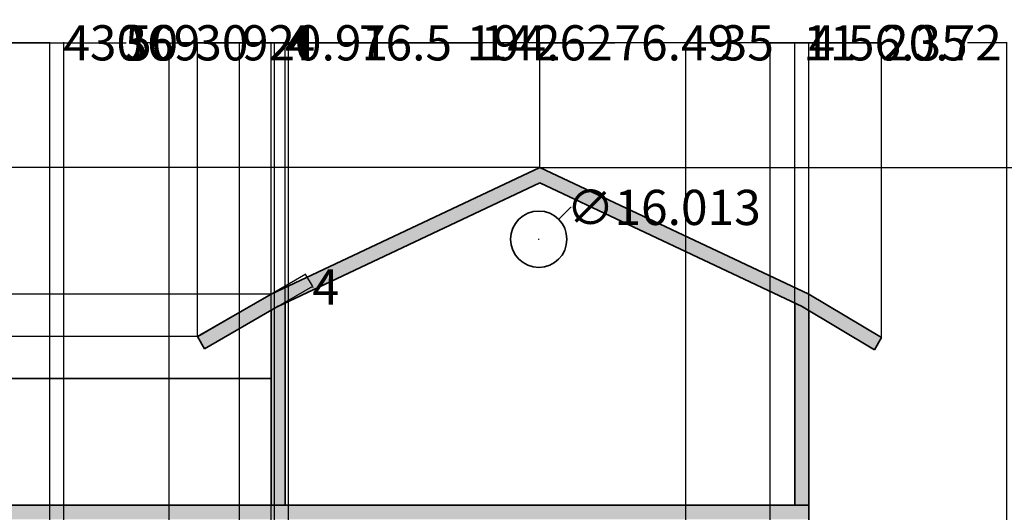
# Model space of a CAD drawing. Units: inches. Extents: x 403 to 1256, y 451 to 842.
# Tile 3 of 4: x 818 to 1098, y 702 to 842. Entities that reach past the tile are written whole.
import ezdxf

# ---------------------------------------------------------------- set-up
doc = ezdxf.new("R2010")
doc.units = ezdxf.units.IN
doc.header["$MEASUREMENT"] = 0
for name, color, linetype, lineweight in [('A-ANNO-DIMS', 2, 'Continuous', 18), ('A-ROOF', 30, 'Continuous', 35), ('A-ROOF-PATT', 30, 'Continuous', 13), ('A-WALL', 7, 'Continuous', 35), ('A-WALL-PATT', 8, 'Continuous', 13)]:
    doc.layers.add(name, color=color, linetype=linetype, lineweight=lineweight)
doc.styles.get("Standard").update_dxf_attribs({"font": 'arial.ttf'})
doc.dimstyles.get("Standard").update_dxf_attribs({"dimtxt": 10, "dimasz": 0.18, "dimexe": 0.18, "dimexo": 0.0625, "dimgap": 0.09, "dimtad": 0, "dimtih": 1, "dimtoh": 1, "dimdec": 0, "dimzin": 0, "dimdsep": 46, "dimlunit": 3, "dimtxsty": 'Standard', "dimcen": 0.09, "dimadec": 0, "dimazin": 0, "dimtfac": 1, "dimtdec": 0, "dimtofl": 0, "dimtmove": 0, "dimatfit": 3, "dimfxl": 1, "dimtolj": 1, "dimtzin": 0, "dimarcsym": 0})

# ---------------------------------------------------------------- blocks, each defined once
blk = doc.blocks.new('*D11')
at = {"layer": 'A-ANNO-DIMS', "color": 0, "lineweight": -2, "transparency": 16777216}
for p, q in [((673.46, 704.02), (673.46, 835.54)), ((673.64, 835.36), (846.82, 835.36)), ((1042.28, 835.36), (869.1, 835.36)), ((1042.46, 704.02), (1042.46, 835.54))]:
    blk.add_line(p, q, dxfattribs=at)
at = {"layer": 'A-ANNO-DIMS', "color": 0, "transparency": 16777216}
for points in [[(673.64, 835.39), (673.64, 835.33), (673.46, 835.36)], [(1042.28, 835.39), (1042.28, 835.33), (1042.46, 835.36)]]:
    blk.add_solid(points, dxfattribs=at)
at = {"layer": 'Defpoints', "color": 0, "transparency": 16777216}
for p in [(1042.46, 835.36), (673.46, 703.96), (1042.46, 703.96)]:
    blk.add_point(p, dxfattribs=at)
at = {"layer": 'A-ANNO-DIMS', "color": 0, "transparency": 16777216, "insert": (857.96, 835.36), "char_height": 10, "attachment_point": 5}
blk.add_mtext('\\A1;369', dxfattribs=at)
blk = doc.blocks.new('*D12')
at = {"layer": 'A-ANNO-DIMS', "color": 0, "lineweight": -2, "transparency": 16777216}
for p, q in [((966.02, 799.96), (1244.44, 799.96)), ((1244.26, 799.78), (1244.26, 632.66)), ((1244.26, 455.14), (1244.26, 622.26)), ((1042.52, 454.96), (1244.44, 454.96))]:
    blk.add_line(p, q, dxfattribs=at)
at = {"layer": 'A-ANNO-DIMS', "color": 0, "transparency": 16777216}
for points in [[(1244.23, 799.78), (1244.29, 799.78), (1244.26, 799.96)], [(1244.23, 455.14), (1244.29, 455.14), (1244.26, 454.96)]]:
    blk.add_solid(points, dxfattribs=at)
at = {"layer": 'Defpoints', "color": 0, "transparency": 16777216}
for p in [(965.96, 799.96), (1244.26, 799.96), (1042.46, 454.96)]:
    blk.add_point(p, dxfattribs=at)
at = {"layer": 'A-ANNO-DIMS', "color": 0, "transparency": 16777216, "insert": (1244.26, 627.46), "char_height": 10, "attachment_point": 5}
blk.add_mtext('\\A1;345', dxfattribs=at)
blk = doc.blocks.new('*D18')
at = {"layer": 'A-ANNO-DIMS', "color": 0, "lineweight": -2, "transparency": 16777216}
for p, q in [((965.9, 799.96), (473.5, 799.96)), ((473.68, 799.78), (473.68, 775.16)), ((473.68, 740.14), (473.68, 764.77)), ((673.4, 739.96), (473.5, 739.96))]:
    blk.add_line(p, q, dxfattribs=at)
at = {"layer": 'A-ANNO-DIMS', "color": 0, "transparency": 16777216}
for points in [[(473.65, 799.78), (473.71, 799.78), (473.68, 799.96)], [(473.65, 740.14), (473.71, 740.14), (473.68, 739.96)]]:
    blk.add_solid(points, dxfattribs=at)
at = {"layer": 'Defpoints', "color": 0, "transparency": 16777216}
for p in [(473.68, 799.96), (965.96, 799.96), (673.46, 739.96)]:
    blk.add_point(p, dxfattribs=at)
at = {"layer": 'A-ANNO-DIMS', "color": 0, "transparency": 16777216, "insert": (473.68, 769.96), "char_height": 10, "attachment_point": 5}
blk.add_mtext('\\A1;60', dxfattribs=at)
blk = doc.blocks.new('*D22')
at = {"layer": 'A-ANNO-DIMS', "color": 0, "lineweight": -2, "transparency": 16777216}
for p, q in [((1007.46, 616.02), (1007.46, 835.54)), ((1007.64, 835.36), (1017.67, 835.36)), ((1042.28, 835.36), (1032.25, 835.36)), ((1042.46, 704.02), (1042.46, 835.54))]:
    blk.add_line(p, q, dxfattribs=at)
at = {"layer": 'A-ANNO-DIMS', "color": 0, "transparency": 16777216}
for points in [[(1007.64, 835.39), (1007.64, 835.33), (1007.46, 835.36)], [(1042.28, 835.39), (1042.28, 835.33), (1042.46, 835.36)]]:
    blk.add_solid(points, dxfattribs=at)
at = {"layer": 'Defpoints', "color": 0, "transparency": 16777216}
for p in [(1042.46, 835.36), (1042.46, 703.96), (1007.46, 615.96)]:
    blk.add_point(p, dxfattribs=at)
at = {"layer": 'A-ANNO-DIMS', "color": 0, "transparency": 16777216, "insert": (1024.96, 835.36), "char_height": 10, "attachment_point": 5}
blk.add_mtext('\\A1;35', dxfattribs=at)
blk = doc.blocks.new('*D23')
at = {"layer": 'A-ANNO-DIMS', "color": 0, "lineweight": -2, "transparency": 16777216}
for p, q in [((682.46, 455.02), (682.46, 835.54)), ((682.64, 835.36), (743.81, 835.36)), ((826.28, 835.36), (765.1, 835.36)), ((826.46, 455.02), (826.46, 835.54))]:
    blk.add_line(p, q, dxfattribs=at)
at = {"layer": 'A-ANNO-DIMS', "color": 0, "transparency": 16777216}
for points in [[(682.64, 835.39), (682.64, 835.33), (682.46, 835.36)], [(826.28, 835.39), (826.28, 835.33), (826.46, 835.36)]]:
    blk.add_solid(points, dxfattribs=at)
at = {"layer": 'Defpoints', "color": 0, "transparency": 16777216}
for p in [(826.46, 835.36), (682.46, 454.96), (826.46, 454.96)]:
    blk.add_point(p, dxfattribs=at)
at = {"layer": 'A-ANNO-DIMS', "color": 0, "transparency": 16777216, "insert": (754.46, 835.36), "char_height": 10, "attachment_point": 5}
blk.add_mtext('\\A1;144', dxfattribs=at)
blk = doc.blocks.new('*D24')
at = {"layer": 'A-ANNO-DIMS', "color": 0, "lineweight": -2, "transparency": 16777216}
for p, q in [((830.46, 539.02), (830.46, 835.54)), ((830.64, 835.36), (848.22, 835.36)), ((880.28, 835.36), (862.69, 835.36)), ((880.46, 539.02), (880.46, 835.54))]:
    blk.add_line(p, q, dxfattribs=at)
at = {"layer": 'A-ANNO-DIMS', "color": 0, "transparency": 16777216}
for points in [[(830.64, 835.39), (830.64, 835.33), (830.46, 835.36)], [(880.28, 835.39), (880.28, 835.33), (880.46, 835.36)]]:
    blk.add_solid(points, dxfattribs=at)
at = {"layer": 'Defpoints', "color": 0, "transparency": 16777216}
for p in [(880.46, 835.36), (830.46, 538.96), (880.46, 538.96)]:
    blk.add_point(p, dxfattribs=at)
at = {"layer": 'A-ANNO-DIMS', "color": 0, "transparency": 16777216, "insert": (855.46, 835.36), "char_height": 10, "attachment_point": 5}
blk.add_mtext('\\A1;50', dxfattribs=at)
blk = doc.blocks.new('*D25')
at = {"layer": 'A-ANNO-DIMS', "color": 0, "lineweight": -2, "transparency": 16777216}
for p, q in [((889.46, 539.02), (889.46, 835.54)), ((889.64, 835.36), (949.84, 835.36)), ((1031.28, 835.36), (971.07, 835.36)), ((1031.46, 539.02), (1031.46, 835.54))]:
    blk.add_line(p, q, dxfattribs=at)
at = {"layer": 'A-ANNO-DIMS', "color": 0, "transparency": 16777216}
for points in [[(889.64, 835.39), (889.64, 835.33), (889.46, 835.36)], [(1031.28, 835.39), (1031.28, 835.33), (1031.46, 835.36)]]:
    blk.add_solid(points, dxfattribs=at)
at = {"layer": 'Defpoints', "color": 0, "transparency": 16777216}
for p in [(1031.46, 835.36), (889.46, 538.96), (1031.46, 538.96)]:
    blk.add_point(p, dxfattribs=at)
at = {"layer": 'A-ANNO-DIMS', "color": 0, "transparency": 16777216, "insert": (960.46, 835.36), "char_height": 10, "attachment_point": 5}
blk.add_mtext('\\A1;142', dxfattribs=at)
blk = doc.blocks.new('*D26')
at = {"layer": 'A-ANNO-DIMS', "color": 0, "lineweight": -2, "transparency": 16777216}
for p, q in [((880.46, 539.02), (880.46, 835.54)), ((880.64, 835.36), (881.58, 835.36)), ((889.28, 835.36), (888.34, 835.36)), ((889.46, 539.02), (889.46, 835.54))]:
    blk.add_line(p, q, dxfattribs=at)
at = {"layer": 'A-ANNO-DIMS', "color": 0, "transparency": 16777216}
for points in [[(880.64, 835.39), (880.64, 835.33), (880.46, 835.36)], [(889.28, 835.39), (889.28, 835.33), (889.46, 835.36)]]:
    blk.add_solid(points, dxfattribs=at)
at = {"layer": 'Defpoints', "color": 0, "transparency": 16777216}
for p in [(889.46, 835.36), (880.46, 538.96), (889.46, 538.96)]:
    blk.add_point(p, dxfattribs=at)
at = {"layer": 'A-ANNO-DIMS', "color": 0, "transparency": 16777216, "insert": (884.96, 835.36), "char_height": 10, "attachment_point": 5}
blk.add_mtext('\\A1;9', dxfattribs=at)
blk = doc.blocks.new('*D27')
at = {"layer": 'A-ANNO-DIMS', "color": 0, "lineweight": -2, "transparency": 16777216}
for p, q in [((1031.46, 455.02), (1031.46, 835.54)), ((1031.64, 835.36), (1042.28, 835.36)), ((1042.46, 455.02), (1042.46, 835.54)), ((1042.46, 835.36), (1042.64, 835.36))]:
    blk.add_line(p, q, dxfattribs=at)
at = {"layer": 'A-ANNO-DIMS', "color": 0, "transparency": 16777216}
for points in [[(1031.64, 835.39), (1031.64, 835.33), (1031.46, 835.36)], [(1042.28, 835.39), (1042.28, 835.33), (1042.46, 835.36)]]:
    blk.add_solid(points, dxfattribs=at)
at = {"layer": 'Defpoints', "color": 0, "transparency": 16777216}
for p in [(1042.46, 835.36), (1031.46, 454.96), (1042.46, 454.96)]:
    blk.add_point(p, dxfattribs=at)
at = {"layer": 'A-ANNO-DIMS', "color": 0, "transparency": 16777216, "insert": (1048.46, 835.36), "char_height": 10, "attachment_point": 5}
blk.add_mtext('\\A1;11', dxfattribs=at)
blk = doc.blocks.new('*D30')
at = {"layer": 'A-ANNO-DIMS', "color": 0, "lineweight": -2, "transparency": 16777216}
for p, q in [((1042.46, 455.02), (1042.46, 835.54)), ((1042.64, 835.36), (1053.63, 835.36)), ((1098.63, 835.36), (1087.63, 835.36)), ((1098.81, 455.02), (1098.81, 835.54))]:
    blk.add_line(p, q, dxfattribs=at)
at = {"layer": 'A-ANNO-DIMS', "color": 0, "transparency": 16777216}
for points in [[(1042.64, 835.39), (1042.64, 835.33), (1042.46, 835.36)], [(1098.63, 835.39), (1098.63, 835.33), (1098.81, 835.36)]]:
    blk.add_solid(points, dxfattribs=at)
at = {"layer": 'Defpoints', "color": 0, "transparency": 16777216}
for p in [(1098.81, 835.36), (1042.46, 454.96), (1098.81, 454.96)]:
    blk.add_point(p, dxfattribs=at)
at = {"layer": 'A-ANNO-DIMS', "color": 0, "transparency": 16777216, "insert": (1070.63, 835.36), "char_height": 10, "attachment_point": 5}
blk.add_mtext('\\A1;56.35', dxfattribs=at)
blk = doc.blocks.new('*D35')
at = {"layer": 'A-ANNO-DIMS', "color": 0, "lineweight": -2, "transparency": 16777216}
for p, q in [((826.46, 616.02), (826.46, 835.54)), ((826.64, 835.36), (830.28, 835.36)), ((830.46, 616.02), (830.46, 835.54)), ((830.46, 835.36), (830.64, 835.36))]:
    blk.add_line(p, q, dxfattribs=at)
at = {"layer": 'A-ANNO-DIMS', "color": 0, "transparency": 16777216}
for points in [[(826.64, 835.39), (826.64, 835.33), (826.46, 835.36)], [(830.28, 835.39), (830.28, 835.33), (830.46, 835.36)]]:
    blk.add_solid(points, dxfattribs=at)
at = {"layer": 'Defpoints', "color": 0, "transparency": 16777216}
for p in [(830.46, 835.36), (826.46, 615.96), (830.46, 615.96)]:
    blk.add_point(p, dxfattribs=at)
at = {"layer": 'A-ANNO-DIMS', "color": 0, "transparency": 16777216, "insert": (834.19, 835.36), "char_height": 10, "attachment_point": 5}
blk.add_mtext('\\A1;4', dxfattribs=at)
blk = doc.blocks.new('*D36')
at = {"layer": 'A-ANNO-DIMS', "color": 0, "lineweight": -2, "transparency": 16777216}
for p, q in [((830.46, 616.02), (830.46, 835.54)), ((830.64, 835.36), (838.23, 835.36)), ((860.28, 835.36), (852.69, 835.36)), ((860.46, 616.02), (860.46, 835.54))]:
    blk.add_line(p, q, dxfattribs=at)
at = {"layer": 'A-ANNO-DIMS', "color": 0, "transparency": 16777216}
for points in [[(830.64, 835.39), (830.64, 835.33), (830.46, 835.36)], [(860.28, 835.39), (860.28, 835.33), (860.46, 835.36)]]:
    blk.add_solid(points, dxfattribs=at)
at = {"layer": 'Defpoints', "color": 0, "transparency": 16777216}
for p in [(860.46, 835.36), (830.46, 615.96), (860.46, 615.96)]:
    blk.add_point(p, dxfattribs=at)
at = {"layer": 'A-ANNO-DIMS', "color": 0, "transparency": 16777216, "insert": (845.46, 835.36), "char_height": 10, "attachment_point": 5}
blk.add_mtext('\\A1;30', dxfattribs=at)
blk = doc.blocks.new('*D37')
at = {"layer": 'A-ANNO-DIMS', "color": 0, "lineweight": -2, "transparency": 16777216}
for p, q in [((860.46, 656.02), (860.46, 835.54)), ((860.64, 835.36), (868.23, 835.36)), ((890.28, 835.36), (882.69, 835.36)), ((890.46, 656.02), (890.46, 835.54))]:
    blk.add_line(p, q, dxfattribs=at)
at = {"layer": 'A-ANNO-DIMS', "color": 0, "transparency": 16777216}
for points in [[(860.64, 835.39), (860.64, 835.33), (860.46, 835.36)], [(890.28, 835.39), (890.28, 835.33), (890.46, 835.36)]]:
    blk.add_solid(points, dxfattribs=at)
at = {"layer": 'Defpoints', "color": 0, "transparency": 16777216}
for p in [(890.46, 835.36), (860.46, 655.96), (890.46, 655.96)]:
    blk.add_point(p, dxfattribs=at)
at = {"layer": 'A-ANNO-DIMS', "color": 0, "transparency": 16777216, "insert": (875.46, 835.36), "char_height": 10, "attachment_point": 5}
blk.add_mtext('\\A1;30', dxfattribs=at)
blk = doc.blocks.new('*D38')
at = {"layer": 'A-ANNO-DIMS', "color": 0, "lineweight": -2, "transparency": 16777216}
for p, q in [((890.46, 616.02), (890.46, 835.54)), ((890.64, 835.36), (894.28, 835.36)), ((894.46, 616.02), (894.46, 835.54)), ((894.46, 835.36), (894.64, 835.36))]:
    blk.add_line(p, q, dxfattribs=at)
at = {"layer": 'A-ANNO-DIMS', "color": 0, "transparency": 16777216}
for points in [[(890.64, 835.39), (890.64, 835.33), (890.46, 835.36)], [(894.28, 835.39), (894.28, 835.33), (894.46, 835.36)]]:
    blk.add_solid(points, dxfattribs=at)
at = {"layer": 'Defpoints', "color": 0, "transparency": 16777216}
for p in [(894.46, 835.36), (890.46, 615.96), (894.46, 615.96)]:
    blk.add_point(p, dxfattribs=at)
at = {"layer": 'A-ANNO-DIMS', "color": 0, "transparency": 16777216, "insert": (898.19, 835.36), "char_height": 10, "attachment_point": 5}
blk.add_mtext('\\A1;4', dxfattribs=at)
blk = doc.blocks.new('*D43')
at = {"layer": 'A-ANNO-DIMS', "color": 0, "lineweight": -2, "transparency": 16777216}
for p, q in [((868.55, 751.96), (868.55, 835.54)), ((868.73, 835.36), (945.54, 835.36)), ((1062.99, 835.36), (986.19, 835.36)), ((1063.17, 751.65), (1063.17, 835.54))]:
    blk.add_line(p, q, dxfattribs=at)
at = {"layer": 'A-ANNO-DIMS', "color": 0, "transparency": 16777216}
for points in [[(868.73, 835.39), (868.73, 835.33), (868.55, 835.36)], [(1062.99, 835.39), (1062.99, 835.33), (1063.17, 835.36)]]:
    blk.add_solid(points, dxfattribs=at)
at = {"layer": 'Defpoints', "color": 0, "transparency": 16777216}
for p in [(1063.17, 835.36), (868.55, 751.9), (1063.17, 751.58)]:
    blk.add_point(p, dxfattribs=at)
at = {"layer": 'A-ANNO-DIMS', "color": 0, "transparency": 16777216, "insert": (965.86, 835.36), "char_height": 10, "attachment_point": 5}
blk.add_mtext('\\A1;194.62', dxfattribs=at)
blk = doc.blocks.new('*D44')
at = {"layer": 'A-ANNO-DIMS', "color": 0, "lineweight": -2, "transparency": 16777216}
for p, q in [((868.55, 751.96), (868.55, 835.54)), ((868.73, 835.36), (889.28, 835.36)), ((889.46, 764.02), (889.46, 835.54)), ((889.46, 835.36), (889.64, 835.36))]:
    blk.add_line(p, q, dxfattribs=at)
at = {"layer": 'A-ANNO-DIMS', "color": 0, "transparency": 16777216}
for points in [[(868.73, 835.39), (868.73, 835.33), (868.55, 835.36)], [(889.28, 835.39), (889.28, 835.33), (889.46, 835.36)]]:
    blk.add_solid(points, dxfattribs=at)
at = {"layer": 'Defpoints', "color": 0, "transparency": 16777216}
for p in [(889.46, 835.36), (889.46, 763.96), (868.55, 751.9)]:
    blk.add_point(p, dxfattribs=at)
at = {"layer": 'A-ANNO-DIMS', "color": 0, "transparency": 16777216, "insert": (905.72, 835.36), "char_height": 10, "attachment_point": 5}
blk.add_mtext('\\A1;20.91', dxfattribs=at)
blk = doc.blocks.new('*D45')
at = {"layer": 'A-ANNO-DIMS', "color": 0, "lineweight": -2, "transparency": 16777216}
for p, q in [((889.46, 764.02), (889.46, 835.54)), ((889.64, 835.36), (914.63, 835.36)), ((965.78, 835.36), (940.78, 835.36)), ((965.96, 800.02), (965.96, 835.54))]:
    blk.add_line(p, q, dxfattribs=at)
at = {"layer": 'A-ANNO-DIMS', "color": 0, "transparency": 16777216}
for points in [[(889.64, 835.39), (889.64, 835.33), (889.46, 835.36)], [(965.78, 835.39), (965.78, 835.33), (965.96, 835.36)]]:
    blk.add_solid(points, dxfattribs=at)
at = {"layer": 'Defpoints', "color": 0, "transparency": 16777216}
for p in [(965.96, 835.36), (965.96, 799.96), (889.46, 763.96)]:
    blk.add_point(p, dxfattribs=at)
at = {"layer": 'A-ANNO-DIMS', "color": 0, "transparency": 16777216, "insert": (927.71, 835.36), "char_height": 10, "attachment_point": 5}
blk.add_mtext('\\A1;76.5', dxfattribs=at)
blk = doc.blocks.new('*D46')
at = {"layer": 'A-ANNO-DIMS', "color": 0, "lineweight": -2, "transparency": 16777216}
for p, q in [((965.96, 800.02), (965.96, 835.54)), ((966.14, 835.36), (987.27, 835.36)), ((1042.27, 835.36), (1021.14, 835.36)), ((1042.45, 764.03), (1042.45, 835.54))]:
    blk.add_line(p, q, dxfattribs=at)
at = {"layer": 'A-ANNO-DIMS', "color": 0, "transparency": 16777216}
for points in [[(966.14, 835.39), (966.14, 835.33), (965.96, 835.36)], [(1042.27, 835.39), (1042.27, 835.33), (1042.45, 835.36)]]:
    blk.add_solid(points, dxfattribs=at)
at = {"layer": 'Defpoints', "color": 0, "transparency": 16777216}
for p in [(1042.45, 835.36), (965.96, 799.96), (1042.45, 763.97)]:
    blk.add_point(p, dxfattribs=at)
at = {"layer": 'A-ANNO-DIMS', "color": 0, "transparency": 16777216, "insert": (1004.2, 835.36), "char_height": 10, "attachment_point": 5}
blk.add_mtext('\\A1;76.49', dxfattribs=at)
blk = doc.blocks.new('*D47')
at = {"layer": 'A-ANNO-DIMS', "color": 0, "lineweight": -2, "transparency": 16777216}
for p, q in [((1042.45, 764.03), (1042.45, 835.54)), ((1042.63, 835.36), (1062.99, 835.36)), ((1063.17, 751.65), (1063.17, 835.54)), ((1063.17, 835.36), (1063.35, 835.36))]:
    blk.add_line(p, q, dxfattribs=at)
at = {"layer": 'A-ANNO-DIMS', "color": 0, "transparency": 16777216}
for points in [[(1042.63, 835.39), (1042.63, 835.33), (1042.45, 835.36)], [(1062.99, 835.39), (1062.99, 835.33), (1063.17, 835.36)]]:
    blk.add_solid(points, dxfattribs=at)
at = {"layer": 'Defpoints', "color": 0, "transparency": 16777216}
for p in [(1063.17, 835.36), (1042.45, 763.97), (1063.17, 751.58)]:
    blk.add_point(p, dxfattribs=at)
at = {"layer": 'A-ANNO-DIMS', "color": 0, "transparency": 16777216, "insert": (1080.35, 835.36), "char_height": 10, "attachment_point": 5}
blk.add_mtext('\\A1;20.72', dxfattribs=at)
blk = doc.blocks.new('*D48')
at = {"layer": 'A-ANNO-DIMS', "color": 0, "lineweight": -2, "transparency": 16777216}
for p, q in [((889.4, 763.96), (473.5, 763.96)), ((473.68, 763.78), (473.68, 763.13)), ((868.49, 751.9), (473.5, 751.9)), ((473.68, 752.08), (473.68, 752.73))]:
    blk.add_line(p, q, dxfattribs=at)
at = {"layer": 'A-ANNO-DIMS', "color": 0, "transparency": 16777216}
for points in [[(473.65, 763.78), (473.71, 763.78), (473.68, 763.96)], [(473.65, 752.08), (473.71, 752.08), (473.68, 751.9)]]:
    blk.add_solid(points, dxfattribs=at)
at = {"layer": 'Defpoints', "color": 0, "transparency": 16777216}
for p in [(473.68, 763.96), (889.46, 763.96), (868.55, 751.9)]:
    blk.add_point(p, dxfattribs=at)
at = {"layer": 'A-ANNO-DIMS', "color": 0, "transparency": 16777216, "insert": (473.68, 757.93), "char_height": 10, "attachment_point": 5}
blk.add_mtext('\\A1;12.062', dxfattribs=at)
blk = doc.blocks.new('*D49')
at = {"layer": 'A-ANNO-DIMS', "color": 0, "lineweight": -2, "transparency": 16777216}
for p, q in [((965.9, 799.96), (473.5, 799.96)), ((473.68, 799.78), (473.68, 787.16)), ((473.68, 764.14), (473.68, 776.76)), ((889.4, 763.96), (473.5, 763.96))]:
    blk.add_line(p, q, dxfattribs=at)
at = {"layer": 'A-ANNO-DIMS', "color": 0, "transparency": 16777216}
for points in [[(473.65, 799.78), (473.71, 799.78), (473.68, 799.96)], [(473.65, 764.14), (473.71, 764.14), (473.68, 763.96)]]:
    blk.add_solid(points, dxfattribs=at)
at = {"layer": 'Defpoints', "color": 0, "transparency": 16777216}
for p in [(473.68, 799.96), (965.96, 799.96), (889.46, 763.96)]:
    blk.add_point(p, dxfattribs=at)
at = {"layer": 'A-ANNO-DIMS', "color": 0, "transparency": 16777216, "insert": (473.68, 781.96), "char_height": 10, "attachment_point": 5}
blk.add_mtext('\\A1;36', dxfattribs=at)
blk = doc.blocks.new('*D50')
at = {"layer": 'A-ANNO-DIMS', "color": 0, "lineweight": -2, "transparency": 16777216}
for p, q in [((868.6, 751.93), (899.37, 769.68)), ((899.3, 769.43), (901.12, 766.28)), ((870.6, 748.47), (901.37, 766.21)), ((901.21, 766.12), (901.3, 765.97)), ((901.3, 765.97), (901.48, 765.97))]:
    blk.add_line(p, q, dxfattribs=at)
at = {"layer": 'A-ANNO-DIMS', "color": 0, "transparency": 16777216}
for points in [[(899.33, 769.45), (899.28, 769.42), (899.21, 769.59)], [(901.15, 766.29), (901.1, 766.26), (901.21, 766.12)]]:
    blk.add_solid(points, dxfattribs=at)
at = {"layer": 'Defpoints', "color": 0, "transparency": 16777216}
for p in [(901.21, 766.12), (868.55, 751.9), (870.55, 748.43)]:
    blk.add_point(p, dxfattribs=at)
at = {"layer": 'A-ANNO-DIMS', "color": 0, "transparency": 16777216, "insert": (905.03, 765.97), "char_height": 10, "attachment_point": 5}
blk.add_mtext('\\A1;4', dxfattribs=at)
blk = doc.blocks.new('*D51')
at = {"layer": 'A-ANNO-DIMS', "color": 0, "lineweight": -2, "transparency": 16777216}
for p, q in [((889.46, 704.02), (889.46, 835.54)), ((889.64, 835.36), (893.28, 835.36)), ((893.46, 704.02), (893.46, 835.54)), ((893.46, 835.36), (893.64, 835.36))]:
    blk.add_line(p, q, dxfattribs=at)
at = {"layer": 'A-ANNO-DIMS', "color": 0, "transparency": 16777216}
for points in [[(889.64, 835.39), (889.64, 835.33), (889.46, 835.36)], [(893.28, 835.39), (893.28, 835.33), (893.46, 835.36)]]:
    blk.add_solid(points, dxfattribs=at)
at = {"layer": 'Defpoints', "color": 0, "transparency": 16777216}
for p in [(893.46, 835.36), (889.46, 703.96), (893.46, 703.96)]:
    blk.add_point(p, dxfattribs=at)
at = {"layer": 'A-ANNO-DIMS', "color": 0, "transparency": 16777216, "insert": (897.19, 835.36), "char_height": 10, "attachment_point": 5}
blk.add_mtext('\\A1;4', dxfattribs=at)
blk = doc.blocks.new('*D52')
at = {"layer": 'A-ANNO-DIMS', "color": 0, "lineweight": -2, "transparency": 16777216}
for p, q in [((1038.46, 704.02), (1038.46, 835.54)), ((1038.64, 835.36), (1042.28, 835.36)), ((1042.46, 704.02), (1042.46, 835.54)), ((1042.46, 835.36), (1042.64, 835.36))]:
    blk.add_line(p, q, dxfattribs=at)
at = {"layer": 'A-ANNO-DIMS', "color": 0, "transparency": 16777216}
for points in [[(1038.64, 835.39), (1038.64, 835.33), (1038.46, 835.36)], [(1042.28, 835.39), (1042.28, 835.33), (1042.46, 835.36)]]:
    blk.add_solid(points, dxfattribs=at)
at = {"layer": 'Defpoints', "color": 0, "transparency": 16777216}
for p in [(1042.46, 835.36), (1038.46, 703.96), (1042.46, 703.96)]:
    blk.add_point(p, dxfattribs=at)
at = {"layer": 'A-ANNO-DIMS', "color": 0, "transparency": 16777216, "insert": (1046.19, 835.36), "char_height": 10, "attachment_point": 5}
blk.add_mtext('\\A1;4', dxfattribs=at)
blk = doc.blocks.new('*D54')
at = {"layer": 'A-ANNO-DIMS', "color": 0, "lineweight": -2, "transparency": 16777216}
for p, q in [((974.69, 788.59), (971.42, 785.33)), ((974.87, 788.59), (974.69, 788.59)), ((965.54, 779.54), (965.72, 779.54)), ((965.63, 779.45), (965.63, 779.63))]:
    blk.add_line(p, q, dxfattribs=at)
at = {"layer": 'A-ANNO-DIMS', "color": 0, "transparency": 16777216}
blk.add_solid([(971.4, 785.35), (971.44, 785.3), (971.29, 785.2)], dxfattribs=at)
at = {"layer": 'Defpoints', "color": 0, "transparency": 16777216}
for p in [(971.29, 785.2), (959.96, 773.89)]:
    blk.add_point(p, dxfattribs=at)
at = {"layer": 'A-ANNO-DIMS', "color": 0, "transparency": 16777216, "insert": (1001.16, 788.59), "char_height": 10, "attachment_point": 5}
blk.add_mtext('\\A1;∅16.013', dxfattribs=at)

msp = doc.modelspace()

# ---------------------------------------------------------------- hatches: boundary and pattern name
at = {"layer": 'A-ROOF-PATT'}
h = msp.add_hatch(color=256, dxfattribs=at)
h.dxf.hatch_style = 1
h.paths.add_polyline_path([(965.959, 795.5407), (1040.5678, 760.4307), (1061.119, 748.15), (1063.1709, 751.5837), (1042.4499, 763.9658), (965.959, 799.9615), (889.459, 763.9615), (868.55, 751.8997), (870.5487, 748.4349), (891.3132, 760.4133)])
at = {"layer": 'A-WALL-PATT'}
h = msp.add_hatch(color=256, dxfattribs=at)
h.dxf.hatch_style = 1
h.paths.add_polyline_path([(893.459, 761.4231), (891.3132, 760.4133), (889.459, 759.3437), (889.459, 703.9615), (893.459, 703.9615)])
h.paths.add_polyline_path([(1042.459, 759.3006), (1040.5678, 760.4307), (1038.459, 761.4231), (1038.459, 703.9615), (1042.459, 703.9615)])
h = msp.add_hatch(dxfattribs=at)
h.set_pattern_fill('AR-CONC', color=256, scale=0.9)
h.set_pattern_definition([(50, (0, 0), (6.455342, -0.56477), [0.675, -7.425]), (355, (0, 0), (-1.248762, 6.76973), [0.54, -5.94]), (100.45144, (0.538, -0.047), (5.20658, 6.20496), [0.573662, -6.31028]), (46.1842, (0, 1.8), (9.60517, -1.489674), [1.0125, -11.1375]), (96.6356, (0.8, 1.676), (8.41196, 8.76707), [0.86049, -9.465424]), (351.1842, (0, 1.8), (8.41196, 8.76707), [0.81, -8.91]), (21, (0.9, 1.35), (5.372163, -3.62357), [0.675, -7.425]), (326, (0.9, 1.35), (2.189838, 6.52635), [0.54, -5.94]), (71.45144, (1.3477, 1.048), (7.562, 2.90278), [0.573662, -6.31028]), (37.5, (0, 0), (0.1094387, 2.9960447), [0, -5.868, 0, -6.03, 0, -5.9625]), (7.5, (0, 0), (2.367626, 3.549705), [0, -3.438, 0, -5.733, 0, -2.2725]), (327.5, (-2.007, 0), (4.804402, -0.202994), [0, -2.25, 0, -7.02, 0, -9.315]), (317.5, (-2.907, 0), (5.248676, 0.900945), [0, -2.925, 0, -4.662, 0, -6.615])])
h.paths.add_polyline_path([(673.459, 703.9615), (673.459, 699.9615), (1033.459, 699.9615), (1042.459, 699.9615), (1042.459, 703.9615), (1033.459, 703.9615)])

# ---------------------------------------------------------------- linework, layer by layer
at = {"layer": 'A-ROOF'}
for p, q in [((965.959, 799.9615), (889.459, 763.9615)), ((965.959, 799.9615), (1042.459, 763.9615)), ((965.959, 795.5407), (891.1622, 760.3422)), ((965.959, 795.5407), (1040.7558, 760.3422)), ((889.459, 763.9615), (868.55, 751.8997)), ((1042.4499, 763.9658), (1063.1709, 751.5837)), ((1042.459, 763.9604), (1042.459, 763.9615)), ((891.4577, 760.4967), (870.5487, 748.4349)), ((1040.3981, 760.5321), (1061.119, 748.15)), ((870.5487, 748.4349), (868.55, 751.8997)), ((1061.119, 748.15), (1063.1709, 751.5837))]:
    msp.add_line(p, q, dxfattribs=at)
msp.add_circle((965.6276, 779.5429), 8.0065, dxfattribs=at)
at = {"layer": 'A-WALL'}
for p, q in [((889.459, 759.3437), (889.459, 703.9615)), ((893.459, 761.4231), (893.459, 703.9615)), ((1038.459, 703.9615), (1038.459, 761.4231)), ((1042.459, 615.9615), (1042.459, 759.3006)), ((673.459, 739.9615), (889.459, 739.9615)), ((673.459, 703.9615), (1033.459, 703.9615)), ((1033.459, 703.9615), (1042.459, 703.9615)), ((1042.459, 703.9615), (1042.459, 699.9615))]:
    msp.add_line(p, q, dxfattribs=at)

# ---------------------------------------------------------------- dimensions: what is measured, and where the dimension line sits
at = {"layer": 'A-ANNO-DIMS'}
for base, p1, p2, override, picture, middle in [((1042.459, 835.3615), (673.459, 703.9615), (1042.459, 703.9615), {"dimdec": 0, "dimlfac": 1, "dimrnd": 0, "dimzin": 0, "dimdsep": 46, "dimlunit": 2}, '*D11', (857.959, 835.3615)), ((826.459, 835.3615), (682.459, 454.9615), (826.459, 454.9615), {"dimdec": 0, "dimlfac": 1, "dimrnd": 0, "dimzin": 0, "dimdsep": 46, "dimlunit": 2}, '*D23', (754.459, 835.3615)), ((830.459, 835.3615), (826.459, 615.9615), (830.459, 615.9615), {"dimdec": 0, "dimlfac": 1, "dimrnd": 0, "dimzin": 0, "dimdsep": 46, "dimlunit": 2}, '*D35', (834.1874, 835.3615)), ((880.459, 835.3615), (830.459, 538.9615), (880.459, 538.9615), {"dimdec": 0, "dimlfac": 1, "dimrnd": 0, "dimzin": 0, "dimdsep": 46, "dimlunit": 2}, '*D24', (855.459, 835.3615)), ((860.459, 835.3615), (830.459, 615.9615), (860.459, 615.9615), {"dimdec": 0, "dimlfac": 1, "dimrnd": 0, "dimzin": 0, "dimdsep": 46, "dimlunit": 2}, '*D36', (845.459, 835.3615)), ((890.459, 835.3615), (860.459, 655.9615), (890.459, 655.9615), {"dimdec": 0, "dimlfac": 1, "dimrnd": 0, "dimzin": 0, "dimdsep": 46, "dimlunit": 2}, '*D37', (875.459, 835.3615)), ((1063.1709, 835.3615), (868.55, 751.8997), (1063.1709, 751.5837), {"dimdec": 2, "dimlfac": 1, "dimrnd": 0, "dimzin": 0, "dimdsep": 46, "dimlunit": 2}, '*D43', (965.8604, 835.3615)), ((889.459, 835.3615), (868.55, 751.8997), (889.459, 763.9615), {"dimdec": 2, "dimlfac": 1, "dimrnd": 0, "dimzin": 0, "dimdsep": 46, "dimlunit": 2}, '*D44', (905.7215, 835.3615)), ((889.459, 835.3615), (880.459, 538.9615), (889.459, 538.9615), {"dimdec": 0, "dimlfac": 1, "dimrnd": 0, "dimzin": 0, "dimdsep": 46, "dimlunit": 2}, '*D26', (884.959, 835.3615)), ((1031.459, 835.3615), (889.459, 538.9615), (1031.459, 538.9615), {"dimdec": 0, "dimlfac": 1, "dimrnd": 0, "dimzin": 0, "dimdsep": 46, "dimlunit": 2}, '*D25', (960.459, 835.3615)), ((965.959, 835.3615), (889.459, 763.9615), (965.959, 799.9615), {"dimdec": 1, "dimlfac": 1, "dimrnd": 0, "dimzin": 0, "dimdsep": 46, "dimlunit": 2}, '*D45', (927.709, 835.3615)), ((893.459, 835.3615), (889.459, 703.9615), (893.459, 703.9615), {"dimdec": 0, "dimlfac": 1, "dimrnd": 0, "dimzin": 0, "dimdsep": 46, "dimlunit": 2}, '*D51', (897.1874, 835.3615)), ((894.459, 835.3615), (890.459, 615.9615), (894.459, 615.9615), {"dimdec": 0, "dimlfac": 1, "dimrnd": 0, "dimzin": 0, "dimdsep": 46, "dimlunit": 2}, '*D38', (898.1874, 835.3615)), ((1042.4499, 835.3615), (965.959, 799.9615), (1042.4499, 763.9658), {"dimdec": 2, "dimlfac": 1, "dimrnd": 0, "dimzin": 0, "dimdsep": 46, "dimlunit": 2}, '*D46', (1004.2045, 835.3615)), ((1042.459, 835.3615), (1007.459, 615.9615), (1042.459, 703.9615), {"dimdec": 0, "dimlfac": 1, "dimrnd": 0, "dimzin": 0, "dimdsep": 46, "dimlunit": 2}, '*D22', (1024.959, 835.3615)), ((1042.459, 835.3615), (1031.459, 454.9615), (1042.459, 454.9615), {"dimdec": 0, "dimlfac": 1, "dimrnd": 0, "dimzin": 0, "dimdsep": 46, "dimlunit": 2}, '*D27', (1048.4555, 835.3615)), ((1042.459, 835.3615), (1038.459, 703.9615), (1042.459, 703.9615), {"dimdec": 0, "dimlfac": 1, "dimrnd": 0, "dimzin": 0, "dimdsep": 46, "dimlunit": 2}, '*D52', (1046.1874, 835.3615)), ((1063.1709, 835.3615), (1042.4499, 763.9658), (1063.1709, 751.5837), {"dimdec": 2, "dimlfac": 1, "dimrnd": 0, "dimzin": 0, "dimdsep": 46, "dimlunit": 2}, '*D47', (1080.3474, 835.3615)), ((1098.8106, 835.3615), (1042.459, 454.9615), (1098.8106, 454.9615), {"dimdec": 2, "dimlfac": 1, "dimrnd": 0, "dimzin": 0, "dimdsep": 46, "dimlunit": 2}, '*D30', (1070.6348, 835.3615))]:
    dim = msp.add_linear_dim(base=base, p1=p1, p2=p2, dimstyle='Standard', override=override, dxfattribs=at)
    dim.commit()
    dim.dimension.update_dxf_attribs({"geometry": picture, "text_midpoint": middle})
for base, p1, p2, angle, override, picture, middle in [((473.6816, 799.9615), (673.459, 739.9615), (965.959, 799.9615), 90, {"dimdec": 0, "dimlfac": 1, "dimrnd": 0, "dimzin": 0, "dimdsep": 46, "dimlunit": 2}, '*D18', (473.6816, 769.9615)), ((473.6816, 799.9615), (889.459, 763.9615), (965.959, 799.9615), 90, {"dimdec": 0, "dimlfac": 1, "dimrnd": 0, "dimzin": 0, "dimdsep": 46, "dimlunit": 2}, '*D49', (473.6816, 781.9615)), ((1244.264, 799.9615), (1042.459, 454.9615), (965.959, 799.9615), 90, {"dimdec": 0, "dimlfac": 1, "dimrnd": 0, "dimzin": 0, "dimdsep": 46, "dimlunit": 2}, '*D12', (1244.264, 627.4615)), ((901.2124, 766.1239), (868.55, 751.8997), (870.5487, 748.4349), 299.979315, {"dimdec": 0, "dimlfac": 1, "dimrnd": 0, "dimzin": 0, "dimdsep": 46, "dimlunit": 2}, '*D50', (905.0308, 765.9679)), ((473.6816, 763.9615), (868.55, 751.8997), (889.459, 763.9615), 90, {"dimdec": 3, "dimlfac": 1, "dimrnd": 0, "dimzin": 0, "dimdsep": 46, "dimlunit": 2}, '*D48', (473.6816, 757.9306))]:
    dim = msp.add_linear_dim(base=base, p1=p1, p2=p2, angle=angle, dimstyle='Standard', override=override, dxfattribs=at)
    dim.commit()
    dim.dimension.update_dxf_attribs({"geometry": picture, "text_midpoint": middle})
dim = msp.add_diameter_dim_2p(p1=(959.9607, 773.8869), p2=(971.2945, 785.1989), dimstyle='Standard', override={"dimdec": 3, "dimlfac": 1, "dimrnd": 0, "dimzin": 0, "dimdsep": 46, "dimlunit": 2}, dxfattribs=at)
dim.commit()
dim.dimension.update_dxf_attribs({"geometry": '*D54', "text_midpoint": (1001.1618, 788.5925), "dimtype": 163})

doc.saveas('drawing.dxf')
